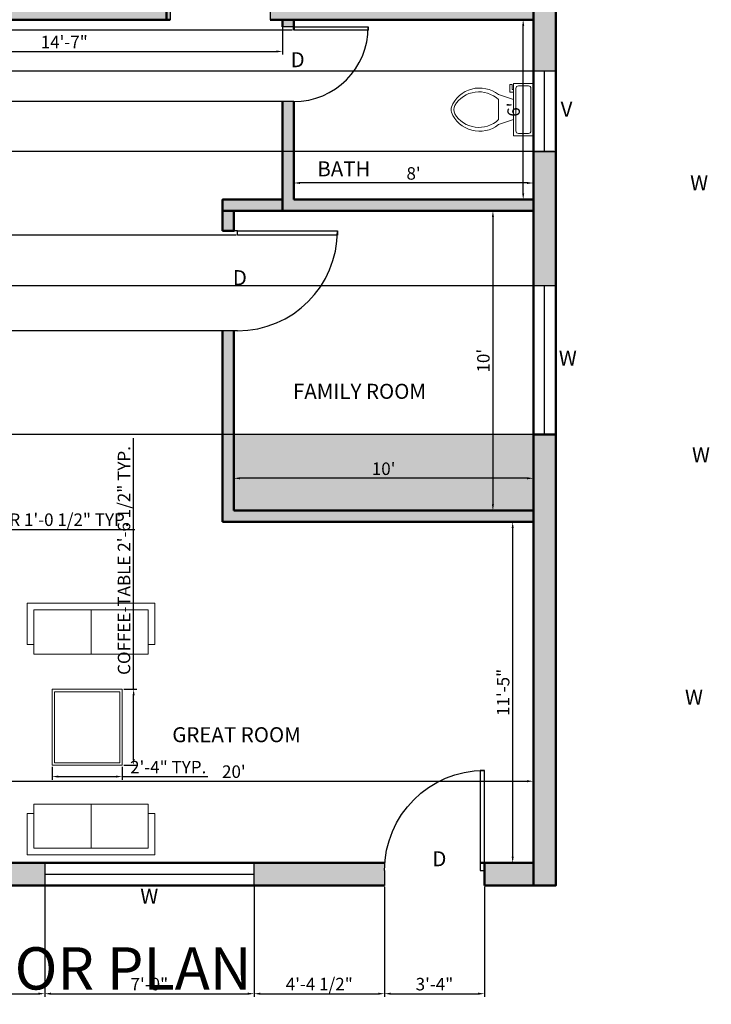
# Model space of a CAD drawing. Units: inches. Extents: x 2064 to 2999, y 1440 to 2089.
# Tile 3 of 7: x 2263 to 2540, y 1440 to 1835. Entities that reach past the tile are written whole.
import ezdxf

# ---------------------------------------------------------------- set-up
doc = ezdxf.new("R2010")
doc.units = ezdxf.units.IN
for name, color, linetype, lineweight in [('A-ANNO-DIMS', 2, 'Continuous', 18), ('A-ANNO-TEXT', 3, 'Continuous', 18), ('A-AREA-IDEN', 7, 'Continuous', 18), ('A-DOOR', 4, 'Continuous', 25), ('A-FLOR-FIXT', 9, 'Continuous', 18), ('A-FURN', 8, 'Continuous', 18), ('A-FURN-PATT', 252, 'Continuous', 13), ('A-GLAZ', 3, 'Continuous', 25), ('A-WALL', 7, 'Continuous', 50), ('A-WALL-PATT', 8, 'Continuous', 13)]:
    doc.layers.add(name, color=color, linetype=linetype, lineweight=lineweight)
doc.styles.get("Standard").update_dxf_attribs({"font": 'arial.ttf'})
doc.dimstyles.new('ISO-25', dxfattribs={"dimtxt": 5, "dimasz": 2.5, "dimexe": 1.25, "dimexo": 0.625, "dimtad": 1, "dimdec": 0, "dimlunit": 4, "dimtxsty": 'Standard', "dimcen": 2.5, "dimadec": 0, "dimazin": 0, "dimtfac": 1, "dimtdec": 0, "dimtmove": 0, "dimatfit": 3, "dimfxl": 1, "dimarcsym": 0})

# ---------------------------------------------------------------- blocks, each defined once
blk = doc.blocks.new('*U2')
for p, q in [((0, 0), (0, -6)), ((40, 0), (40, -6))]:
    blk.add_line(p, q)
blk.add_lwpolyline([(0, 0), (0, 40), (1.75, 40), (1.75, 0)], close=True)
blk.add_arc((0, 0), 40, 0, 90)
blk = doc.blocks.new('*U4')
for p, q in [((9.5, -6), (9.5, -2)), ((-10, -8.5), (-8, -8.5)), ((-10, -9.5), (-10, -8.5)), ((-7, -9.5), (-10, -9.5)), ((-8, -8.5), (-8, -8)), ((-7, -8), (-7, -9.5)), ((-4, -8), (-6, -14)), ((4, -8), (6, -14)), ((4, -14), (-4, -14))]:
    blk.add_line(p, q)
blk.add_lwpolyline([(10.5, -8), (10.5, 0), (-10.5, 0), (-10.5, -8)], close=True)
for points in [[(-9.5, -2), (-9.5, -6)], [(8.5, -1), (-8.5, -1)], [(-8.5, -7), (8.5, -7)]]:
    blk.add_lwpolyline(points)
for centre, radius, start, end in [((-8.62, -1.88), 0.884, 81.8699, 188.1301), ((8.62, -1.88), 0.884, 351.8699, 98.1301), ((-8.62, -6.12), 0.884, 171.8699, 278.1301), ((8.62, -6.12), 0.884, 261.8699, 8.1301), ((3.52, -21.58), 12.17, 141.4691, 247.9714), ((4.2, -21.82), 11.33, 136.3677, 238.9468), ((-3.52, -21.58), 12.17, 292.0284, 38.5307), ((-4.2, -21.82), 11.33, 301.053, 43.6321), ((0, -27.88), 4, 245.7318, 294.2682), ((0, -29), 4, 254.8605, 285.1395)]:
    blk.add_arc(centre, radius, start, end)
blk = doc.blocks.new('*D10')
at = {"layer": 'A-ANNO-DIMS', "color": 0, "lineweight": -2, "transparency": 16777216}
for p, q in [((2468.19, 1834.57), (2463.48, 1834.57)), ((2464.73, 1765.07), (2464.73, 1832.07)), ((2468.19, 1762.57), (2463.48, 1762.57))]:
    blk.add_line(p, q, dxfattribs=at)
at = {"layer": 'A-ANNO-DIMS', "color": 0, "transparency": 16777216}
for points in [[(2464.32, 1832.07), (2465.15, 1832.07), (2464.73, 1834.57)], [(2464.32, 1765.07), (2465.15, 1765.07), (2464.73, 1762.57)]]:
    blk.add_solid(points, dxfattribs=at)
at = {"layer": 'Defpoints', "color": 0, "transparency": 16777216}
for p in [(2464.73, 1834.57), (2468.82, 1834.57), (2468.82, 1762.57)]:
    blk.add_point(p, dxfattribs=at)
at = {"layer": 'A-ANNO-DIMS', "color": 0, "transparency": 16777216, "insert": (2461.55, 1798.57), "char_height": 5, "attachment_point": 5, "rotation": 90}
blk.add_mtext("6'", dxfattribs=at)
blk = doc.blocks.new('*D11')
at = {"layer": 'A-ANNO-DIMS', "color": 0, "lineweight": -2, "transparency": 16777216}
for p, q in [((2372.82, 1763.2), (2372.82, 1770.46)), ((2468.82, 1763.2), (2468.82, 1770.46)), ((2466.32, 1769.21), (2375.32, 1769.21))]:
    blk.add_line(p, q, dxfattribs=at)
at = {"layer": 'A-ANNO-DIMS', "color": 0, "transparency": 16777216}
for points in [[(2375.32, 1769.63), (2375.32, 1768.8), (2372.82, 1769.21)], [(2466.32, 1769.63), (2466.32, 1768.8), (2468.82, 1769.21)]]:
    blk.add_solid(points, dxfattribs=at)
at = {"layer": 'Defpoints', "color": 0, "transparency": 16777216}
for p in [(2372.82, 1769.21), (2372.82, 1762.57), (2468.82, 1762.57)]:
    blk.add_point(p, dxfattribs=at)
at = {"layer": 'A-ANNO-DIMS', "color": 0, "transparency": 16777216, "insert": (2420.82, 1772.39), "char_height": 5, "attachment_point": 5}
blk.add_mtext("8'", dxfattribs=at)
blk = doc.blocks.new('*D12')
at = {"layer": 'A-ANNO-DIMS', "color": 0, "lineweight": -2, "transparency": 16777216}
for p, q in [((2348.82, 1638.7), (2348.82, 1652.27)), ((2468.82, 1638.7), (2468.82, 1652.27)), ((2466.32, 1651.02), (2351.32, 1651.02))]:
    blk.add_line(p, q, dxfattribs=at)
at = {"layer": 'A-ANNO-DIMS', "color": 0, "transparency": 16777216}
for points in [[(2351.32, 1651.43), (2351.32, 1650.6), (2348.82, 1651.02)], [(2466.32, 1651.43), (2466.32, 1650.6), (2468.82, 1651.02)]]:
    blk.add_solid(points, dxfattribs=at)
at = {"layer": 'Defpoints', "color": 0, "transparency": 16777216}
for p in [(2348.82, 1651.02), (2348.82, 1638.07), (2468.82, 1638.07)]:
    blk.add_point(p, dxfattribs=at)
at = {"layer": 'A-ANNO-DIMS', "color": 0, "transparency": 16777216, "insert": (2408.82, 1654.19), "char_height": 5, "attachment_point": 5}
blk.add_mtext("10'", dxfattribs=at)
blk = doc.blocks.new('*D13')
at = {"layer": 'A-ANNO-DIMS', "color": 0, "lineweight": -2, "transparency": 16777216}
for p, q in [((2468.19, 1758.07), (2451.35, 1758.07)), ((2452.6, 1755.57), (2452.6, 1640.57)), ((2468.19, 1638.07), (2451.35, 1638.07))]:
    blk.add_line(p, q, dxfattribs=at)
at = {"layer": 'A-ANNO-DIMS', "color": 0, "transparency": 16777216}
for points in [[(2452.19, 1755.57), (2453.02, 1755.57), (2452.6, 1758.07)], [(2452.19, 1640.57), (2453.02, 1640.57), (2452.6, 1638.07)]]:
    blk.add_solid(points, dxfattribs=at)
at = {"layer": 'Defpoints', "color": 0, "transparency": 16777216}
for p in [(2468.82, 1758.07), (2452.6, 1638.07), (2468.82, 1638.07)]:
    blk.add_point(p, dxfattribs=at)
at = {"layer": 'A-ANNO-DIMS', "color": 0, "transparency": 16777216, "insert": (2449.43, 1698.07), "char_height": 5, "attachment_point": 5, "rotation": 90}
blk.add_mtext("10'", dxfattribs=at)
blk = doc.blocks.new('*D15')
at = {"layer": 'A-ANNO-DIMS', "color": 0, "lineweight": -2, "transparency": 16777216}
for p, q in [((2228.82, 1497.7), (2228.82, 1531.02)), ((2231.32, 1529.77), (2466.32, 1529.77)), ((2468.82, 1497.7), (2468.82, 1531.02))]:
    blk.add_line(p, q, dxfattribs=at)
at = {"layer": 'A-ANNO-DIMS', "color": 0, "transparency": 16777216}
for points in [[(2231.32, 1530.19), (2231.32, 1529.36), (2228.82, 1529.77)], [(2466.32, 1530.19), (2466.32, 1529.36), (2468.82, 1529.77)]]:
    blk.add_solid(points, dxfattribs=at)
at = {"layer": 'Defpoints', "color": 0, "transparency": 16777216}
for p in [(2468.82, 1529.77), (2228.82, 1497.07), (2468.82, 1497.07)]:
    blk.add_point(p, dxfattribs=at)
at = {"layer": 'A-ANNO-DIMS', "color": 0, "transparency": 16777216, "insert": (2348.82, 1532.95), "char_height": 5, "attachment_point": 5}
blk.add_mtext("20'", dxfattribs=at)
blk = doc.blocks.new('*D16')
at = {"layer": 'A-ANNO-DIMS', "color": 0, "lineweight": -2, "transparency": 16777216}
for p, q in [((2193.43, 1833.95), (2193.43, 1820.6)), ((2368.32, 1833.95), (2368.32, 1820.6)), ((2195.93, 1821.85), (2365.82, 1821.85))]:
    blk.add_line(p, q, dxfattribs=at)
at = {"layer": 'A-ANNO-DIMS', "color": 0, "transparency": 16777216}
for points in [[(2195.93, 1822.26), (2195.93, 1821.43), (2193.43, 1821.85)], [(2365.82, 1822.26), (2365.82, 1821.43), (2368.32, 1821.85)]]:
    blk.add_solid(points, dxfattribs=at)
at = {"layer": 'Defpoints', "color": 0, "transparency": 16777216}
for p in [(2193.43, 1834.57), (2368.32, 1834.57), (2368.32, 1821.85)]:
    blk.add_point(p, dxfattribs=at)
at = {"layer": 'A-ANNO-DIMS', "color": 0, "transparency": 16777216, "insert": (2280.88, 1824.98), "char_height": 5, "attachment_point": 5}
blk.add_mtext('14\'-7"', dxfattribs=at)
blk = doc.blocks.new('*D38')
at = {"layer": 'A-ANNO-DIMS', "color": 0, "lineweight": -2, "transparency": 16777216}
for p, q in [((2468.19, 1633.57), (2459.27, 1633.57)), ((2460.52, 1499.57), (2460.52, 1631.07)), ((2468.19, 1497.07), (2459.27, 1497.07))]:
    blk.add_line(p, q, dxfattribs=at)
at = {"layer": 'A-ANNO-DIMS', "color": 0, "transparency": 16777216}
for points in [[(2460.11, 1631.07), (2460.94, 1631.07), (2460.52, 1633.57)], [(2460.11, 1499.57), (2460.94, 1499.57), (2460.52, 1497.07)]]:
    blk.add_solid(points, dxfattribs=at)
at = {"layer": 'Defpoints', "color": 0, "transparency": 16777216}
for p in [(2460.52, 1633.57), (2468.82, 1633.57), (2468.82, 1497.07)]:
    blk.add_point(p, dxfattribs=at)
at = {"layer": 'A-ANNO-DIMS', "color": 0, "transparency": 16777216, "insert": (2457.35, 1565.32), "char_height": 5, "attachment_point": 5, "rotation": 90}
blk.add_mtext('11\'-5"', dxfattribs=at)
blk = doc.blocks.new('SOFA-2')
for p, q in [((25.58, 20.31), (25.58, 2.6)), ((2.71, 16.54), (0, 16.54)), ((0, 16.54), (0, 0)), ((51.13, 16.54), (48.46, 16.54)), ((51.13, 0), (51.13, 16.54)), ((0, 0), (51.13, 0))]:
    blk.add_line(p, q)
blk.add_lwpolyline([(2.71, 2.6), (48.46, 2.6), (48.46, 20.31), (2.71, 20.31)], close=True)
blk = doc.blocks.new('COFFEE-TABLE')
for points in [[(0, 0), (28.15, 0), (28.15, 30.4), (0, 30.4)], [(1, 1), (27.15, 1), (27.15, 29.4), (1, 29.4)]]:
    blk.add_lwpolyline(points, close=True)
blk = doc.blocks.new('WIN-60')
blk.add_line((4.5, 0), (4.5, 59.54))
blk.add_lwpolyline([(0, 0), (9, 0), (9, 59.54), (0, 59.54)], close=True)
blk = doc.blocks.new('*D55')
at = {"layer": 'A-ANNO-DIMS', "color": 0, "lineweight": -2, "transparency": 16777216}
for p, q in [((2308.68, 1566.59), (2308.68, 1667.13)), ((2304.75, 1566.59), (2309.93, 1566.59)), ((2308.68, 1538.68), (2308.68, 1564.09)), ((2304.75, 1536.18), (2309.93, 1536.18))]:
    blk.add_line(p, q, dxfattribs=at)
at = {"layer": 'A-ANNO-DIMS', "color": 0, "transparency": 16777216}
for points in [[(2308.27, 1564.09), (2309.1, 1564.09), (2308.68, 1566.59)], [(2308.27, 1538.68), (2309.1, 1538.68), (2308.68, 1536.18)]]:
    blk.add_solid(points, dxfattribs=at)
at = {"layer": 'Defpoints', "color": 0, "transparency": 16777216}
for p in [(2304.12, 1566.59), (2308.68, 1566.59), (2304.12, 1536.18)]:
    blk.add_point(p, dxfattribs=at)
at = {"layer": 'A-ANNO-DIMS', "color": 0, "transparency": 16777216, "insert": (2305.47, 1618.11), "char_height": 5, "attachment_point": 5, "rotation": 90}
blk.add_mtext('COFFEE-TABLE 2\'-6 1/2" TYP.', dxfattribs=at)
blk = doc.blocks.new('*D56')
at = {"layer": 'A-ANNO-DIMS', "color": 0, "lineweight": -2, "transparency": 16777216}
for p, q in [((2275.98, 1535.56), (2275.98, 1530.37)), ((2304.12, 1535.56), (2304.12, 1530.37)), ((2278.48, 1531.62), (2301.62, 1531.62)), ((2304.12, 1531.62), (2338.44, 1531.62))]:
    blk.add_line(p, q, dxfattribs=at)
at = {"layer": 'A-ANNO-DIMS', "color": 0, "transparency": 16777216}
for points in [[(2278.48, 1532.04), (2278.48, 1531.21), (2275.98, 1531.62)], [(2301.62, 1532.04), (2301.62, 1531.21), (2304.12, 1531.62)]]:
    blk.add_solid(points, dxfattribs=at)
at = {"layer": 'Defpoints', "color": 0, "transparency": 16777216}
for p in [(2275.98, 1536.18), (2304.12, 1536.18), (2304.12, 1531.62)]:
    blk.add_point(p, dxfattribs=at)
at = {"layer": 'A-ANNO-DIMS', "color": 0, "transparency": 16777216, "insert": (2322.53, 1534.76), "char_height": 5, "attachment_point": 5}
blk.add_mtext('2\'-4" TYP.', dxfattribs=at)
blk = doc.blocks.new('*D57')
at = {"layer": 'A-ANNO-DIMS', "color": 0, "lineweight": -2, "transparency": 16777216}
for p, q in [((2200.61, 1631.83), (2200.61, 1629.33)), ((2213.15, 1631.83), (2213.15, 1629.33)), ((2203.11, 1630.58), (2210.65, 1630.58)), ((2213.15, 1630.58), (2309.22, 1630.58))]:
    blk.add_line(p, q, dxfattribs=at)
at = {"layer": 'A-ANNO-DIMS', "color": 0, "transparency": 16777216}
for points in [[(2203.11, 1631), (2203.11, 1630.16), (2200.61, 1630.58)], [(2210.65, 1631), (2210.65, 1630.16), (2213.15, 1630.58)]]:
    blk.add_solid(points, dxfattribs=at)
at = {"layer": 'Defpoints', "color": 0, "transparency": 16777216}
for p in [(2200.61, 1632.46), (2213.15, 1632.46), (2213.15, 1630.58)]:
    blk.add_point(p, dxfattribs=at)
at = {"layer": 'A-ANNO-DIMS', "color": 0, "transparency": 16777216, "insert": (2262.43, 1633.79), "char_height": 5, "attachment_point": 5}
blk.add_mtext('DINING-CHAIR 1\'-0 1/2" TYP.', dxfattribs=at)
blk = doc.blocks.new('*D70')
at = {"layer": 'A-ANNO-DIMS', "color": 0, "lineweight": -2, "transparency": 16777216}
for p, q in [((2477.19, 1865.66), (2073.22, 1865.66)), ((2074.47, 1863.16), (2074.47, 1816.51)), ((2477.19, 1814.01), (2073.22, 1814.01))]:
    blk.add_line(p, q, dxfattribs=at)
at = {"layer": 'A-ANNO-DIMS', "color": 0, "transparency": 16777216}
for points in [[(2074.05, 1863.16), (2074.89, 1863.16), (2074.47, 1865.66)], [(2074.05, 1816.51), (2074.89, 1816.51), (2074.47, 1814.01)]]:
    blk.add_solid(points, dxfattribs=at)
at = {"layer": 'Defpoints', "color": 0, "transparency": 16777216}
for p in [(2477.82, 1865.66), (2074.47, 1814.01), (2477.82, 1814.01)]:
    blk.add_point(p, dxfattribs=at)
at = {"layer": 'A-ANNO-DIMS', "color": 0, "transparency": 16777216, "insert": (2071.26, 1839.83), "char_height": 5, "attachment_point": 5, "rotation": 90}
blk.add_mtext('4\'-3 1/2"', dxfattribs=at)
blk = doc.blocks.new('*D71')
at = {"layer": 'A-ANNO-DIMS', "color": 0, "lineweight": -2, "transparency": 16777216}
for p, q in [((2477.19, 1814.01), (2073.22, 1814.01)), ((2074.47, 1811.51), (2074.47, 1784.3)), ((2477.19, 1781.8), (2073.22, 1781.8))]:
    blk.add_line(p, q, dxfattribs=at)
at = {"layer": 'A-ANNO-DIMS', "color": 0, "transparency": 16777216}
for points in [[(2074.05, 1811.51), (2074.89, 1811.51), (2074.47, 1814.01)], [(2074.05, 1784.3), (2074.89, 1784.3), (2074.47, 1781.8)]]:
    blk.add_solid(points, dxfattribs=at)
at = {"layer": 'Defpoints', "color": 0, "transparency": 16777216}
for p in [(2477.82, 1814.01), (2074.47, 1781.8), (2477.82, 1781.8)]:
    blk.add_point(p, dxfattribs=at)
at = {"layer": 'A-ANNO-DIMS', "color": 0, "transparency": 16777216, "insert": (2071.29, 1797.91), "char_height": 5, "attachment_point": 5, "rotation": 90}
blk.add_mtext('2\'-8"', dxfattribs=at)
blk = doc.blocks.new('*D72')
at = {"layer": 'A-ANNO-DIMS', "color": 0, "lineweight": -2, "transparency": 16777216}
for p, q in [((2477.19, 1781.8), (2073.22, 1781.8)), ((2074.47, 1779.3), (2074.47, 1730.57)), ((2477.19, 1728.07), (2073.22, 1728.07))]:
    blk.add_line(p, q, dxfattribs=at)
at = {"layer": 'A-ANNO-DIMS', "color": 0, "transparency": 16777216}
for points in [[(2074.05, 1779.3), (2074.89, 1779.3), (2074.47, 1781.8)], [(2074.05, 1730.57), (2074.89, 1730.57), (2074.47, 1728.07)]]:
    blk.add_solid(points, dxfattribs=at)
at = {"layer": 'Defpoints', "color": 0, "transparency": 16777216}
for p in [(2477.82, 1781.8), (2074.47, 1728.07), (2477.82, 1728.07)]:
    blk.add_point(p, dxfattribs=at)
at = {"layer": 'A-ANNO-DIMS', "color": 0, "transparency": 16777216, "insert": (2071.26, 1754.94), "char_height": 5, "attachment_point": 5, "rotation": 90}
blk.add_mtext('4\'-5 1/2"', dxfattribs=at)
blk = doc.blocks.new('*D73')
at = {"layer": 'A-ANNO-DIMS', "color": 0, "lineweight": -2, "transparency": 16777216}
for p, q in [((2477.19, 1728.07), (2073.22, 1728.07)), ((2074.47, 1725.57), (2074.47, 1671.03)), ((2477.19, 1668.53), (2073.22, 1668.53))]:
    blk.add_line(p, q, dxfattribs=at)
at = {"layer": 'A-ANNO-DIMS', "color": 0, "transparency": 16777216}
for points in [[(2074.05, 1725.57), (2074.89, 1725.57), (2074.47, 1728.07)], [(2074.05, 1671.03), (2074.89, 1671.03), (2074.47, 1668.53)]]:
    blk.add_solid(points, dxfattribs=at)
at = {"layer": 'Defpoints', "color": 0, "transparency": 16777216}
for p in [(2477.82, 1728.07), (2074.47, 1668.53), (2477.82, 1668.53)]:
    blk.add_point(p, dxfattribs=at)
at = {"layer": 'A-ANNO-DIMS', "color": 0, "transparency": 16777216, "insert": (2071.26, 1698.3), "char_height": 5, "attachment_point": 5, "rotation": 90}
blk.add_mtext('4\'-11 1/2"', dxfattribs=at)
blk = doc.blocks.new('*D78')
at = {"layer": 'A-ANNO-DIMS', "color": 0, "lineweight": -2, "transparency": 16777216}
for p, q in [((2117.82, 1487.45), (2117.82, 1443.47)), ((2273.05, 1487.45), (2273.05, 1443.47)), ((2120.32, 1444.72), (2270.55, 1444.72))]:
    blk.add_line(p, q, dxfattribs=at)
at = {"layer": 'A-ANNO-DIMS', "color": 0, "transparency": 16777216}
for points in [[(2120.32, 1445.14), (2120.32, 1444.3), (2117.82, 1444.72)], [(2270.55, 1445.14), (2270.55, 1444.3), (2273.05, 1444.72)]]:
    blk.add_solid(points, dxfattribs=at)
at = {"layer": 'Defpoints', "color": 0, "transparency": 16777216}
for p in [(2117.82, 1488.07), (2273.05, 1488.07), (2273.05, 1444.72)]:
    blk.add_point(p, dxfattribs=at)
at = {"layer": 'A-ANNO-DIMS', "color": 0, "transparency": 16777216, "insert": (2195.43, 1447.86), "char_height": 5, "attachment_point": 5}
blk.add_mtext('12\'-11"', dxfattribs=at)
blk = doc.blocks.new('*D79')
at = {"layer": 'A-ANNO-DIMS', "color": 0, "lineweight": -2, "transparency": 16777216}
for p, q in [((2273.05, 1487.45), (2273.05, 1443.47)), ((2356.92, 1487.45), (2356.92, 1443.47)), ((2275.55, 1444.72), (2354.42, 1444.72))]:
    blk.add_line(p, q, dxfattribs=at)
at = {"layer": 'A-ANNO-DIMS', "color": 0, "transparency": 16777216}
for points in [[(2275.55, 1445.14), (2275.55, 1444.3), (2273.05, 1444.72)], [(2354.42, 1445.14), (2354.42, 1444.3), (2356.92, 1444.72)]]:
    blk.add_solid(points, dxfattribs=at)
at = {"layer": 'Defpoints', "color": 0, "transparency": 16777216}
for p in [(2273.05, 1488.07), (2356.92, 1488.07), (2356.92, 1444.72)]:
    blk.add_point(p, dxfattribs=at)
at = {"layer": 'A-ANNO-DIMS', "color": 0, "transparency": 16777216, "insert": (2314.98, 1447.9), "char_height": 5, "attachment_point": 5}
blk.add_mtext('7\'-0"', dxfattribs=at)
blk = doc.blocks.new('*D80')
at = {"layer": 'A-ANNO-DIMS', "color": 0, "lineweight": -2, "transparency": 16777216}
for p, q in [((2356.92, 1487.45), (2356.92, 1443.47)), ((2409.19, 1487.45), (2409.19, 1443.47)), ((2359.42, 1444.72), (2406.69, 1444.72))]:
    blk.add_line(p, q, dxfattribs=at)
at = {"layer": 'A-ANNO-DIMS', "color": 0, "transparency": 16777216}
for points in [[(2359.42, 1445.14), (2359.42, 1444.3), (2356.92, 1444.72)], [(2406.69, 1445.14), (2406.69, 1444.3), (2409.19, 1444.72)]]:
    blk.add_solid(points, dxfattribs=at)
at = {"layer": 'Defpoints', "color": 0, "transparency": 16777216}
for p in [(2356.92, 1488.07), (2409.19, 1488.07), (2409.19, 1444.72)]:
    blk.add_point(p, dxfattribs=at)
at = {"layer": 'A-ANNO-DIMS', "color": 0, "transparency": 16777216, "insert": (2383.05, 1447.93), "char_height": 5, "attachment_point": 5}
blk.add_mtext('4\'-4 1/2"', dxfattribs=at)
blk = doc.blocks.new('*D81')
at = {"layer": 'A-ANNO-DIMS', "color": 0, "lineweight": -2, "transparency": 16777216}
for p, q in [((2409.19, 1487.45), (2409.19, 1443.47)), ((2449.19, 1487.45), (2449.19, 1443.47)), ((2411.69, 1444.72), (2446.69, 1444.72))]:
    blk.add_line(p, q, dxfattribs=at)
at = {"layer": 'A-ANNO-DIMS', "color": 0, "transparency": 16777216}
for points in [[(2411.69, 1445.14), (2411.69, 1444.3), (2409.19, 1444.72)], [(2446.69, 1445.14), (2446.69, 1444.3), (2449.19, 1444.72)]]:
    blk.add_solid(points, dxfattribs=at)
at = {"layer": 'Defpoints', "color": 0, "transparency": 16777216}
for p in [(2409.19, 1488.07), (2449.19, 1488.07), (2449.19, 1444.72)]:
    blk.add_point(p, dxfattribs=at)
at = {"layer": 'A-ANNO-DIMS', "color": 0, "transparency": 16777216, "insert": (2429.19, 1447.9), "char_height": 5, "attachment_point": 5}
blk.add_mtext('3\'-4"', dxfattribs=at)
blk = doc.blocks.new('*D113')
at = {"layer": 'A-ANNO-DIMS', "color": 0, "lineweight": -2, "transparency": 16777216}
for p, q in [((2372.19, 1830.37), (2073.22, 1830.37)), ((2074.47, 1827.87), (2074.47, 1804.28)), ((2372.19, 1801.78), (2073.22, 1801.78))]:
    blk.add_line(p, q, dxfattribs=at)
at = {"layer": 'A-ANNO-DIMS', "color": 0, "transparency": 16777216}
for points in [[(2074.05, 1827.87), (2074.89, 1827.87), (2074.47, 1830.37)], [(2074.05, 1804.28), (2074.89, 1804.28), (2074.47, 1801.78)]]:
    blk.add_solid(points, dxfattribs=at)
at = {"layer": 'Defpoints', "color": 0, "transparency": 16777216}
for p in [(2372.82, 1830.37), (2074.47, 1801.78), (2372.82, 1801.78)]:
    blk.add_point(p, dxfattribs=at)
at = {"layer": 'A-ANNO-DIMS', "color": 0, "transparency": 16777216, "insert": (2071.26, 1816.07), "char_height": 5, "attachment_point": 5, "rotation": 90}
blk.add_mtext('2\'-4 1/2"', dxfattribs=at)
blk = doc.blocks.new('*D114')
at = {"layer": 'A-ANNO-DIMS', "color": 0, "lineweight": -2, "transparency": 16777216}
for p, q in [((2349.69, 1748.3), (2073.22, 1748.3)), ((2074.47, 1745.8), (2074.47, 1712.55)), ((2348.19, 1710.05), (2073.22, 1710.05))]:
    blk.add_line(p, q, dxfattribs=at)
at = {"layer": 'A-ANNO-DIMS', "color": 0, "transparency": 16777216}
for points in [[(2074.05, 1745.8), (2074.89, 1745.8), (2074.47, 1748.3)], [(2074.05, 1712.55), (2074.89, 1712.55), (2074.47, 1710.05)]]:
    blk.add_solid(points, dxfattribs=at)
at = {"layer": 'Defpoints', "color": 0, "transparency": 16777216}
for p in [(2350.32, 1748.3), (2074.47, 1710.05), (2348.82, 1710.05)]:
    blk.add_point(p, dxfattribs=at)
at = {"layer": 'A-ANNO-DIMS', "color": 0, "transparency": 16777216, "insert": (2071.26, 1729.18), "char_height": 5, "attachment_point": 5, "rotation": 90}
blk.add_mtext('3\'-2 1/2"', dxfattribs=at)

msp = doc.modelspace()

# ---------------------------------------------------------------- hatches: boundary and pattern name
at = {"layer": 'A-FURN-PATT'}
h = msp.add_hatch(color=256, dxfattribs=at)
h.dxf.hatch_style = 1
h.paths.add_polyline_path([(2211.98, 1959.07), (2126.82, 1959.07), (2126.82, 1938.57), (2211.98, 1938.57)])
h.paths.add_polyline_path([(2669.87, 1959.07), (2646.96, 1959.07), (2646.96, 1892.49), (2669.87, 1892.49)])
h.paths.add_polyline_path([(2468.82, 1668.53), (2348.82, 1668.53), (2348.82, 1638.07), (2468.82, 1638.07)])
h.paths.add_polyline_path([(2891.87, 1667.99), (2780.13, 1667.99), (2780.13, 1638.07), (2891.87, 1638.07)])
h.paths.add_polyline_path([(2854.27, 1658.75), (2854.27, 1650.97), (2859.31, 1650.97), (2859.31, 1658.75), (2862.16, 1658.75), (2862.16, 1650.97), (2867.47, 1650.97), (2867.47, 1658.75), (2870.33, 1658.75), (2870.33, 1650.97), (2879.45, 1650.97), (2879.45, 1658.75), (2882.31, 1658.75), (2882.31, 1643.24), (2879.45, 1643.24), (2879.45, 1650.97), (2870.33, 1650.97), (2870.33, 1643.24), (2867.47, 1643.24), (2867.47, 1650.97), (2862.16, 1650.97), (2862.16, 1643.24), (2859.31, 1643.24), (2859.31, 1650.97), (2854.27, 1650.97), (2854.27, 1643.24), (2851.41, 1643.24), (2851.41, 1650.97), (2845.97, 1650.97), (2845.97, 1643.24), (2843.11, 1643.24), (2843.11, 1650.97), (2839.98, 1650.97), (2839.98, 1643.24), (2837.12, 1643.24), (2837.12, 1650.97), (2831.27, 1650.97), (2831.27, 1643.24), (2828.41, 1643.24), (2828.41, 1650.97), (2823.78, 1650.97), (2823.78, 1643.24), (2820.92, 1643.24), (2820.92, 1650.97), (2816.56, 1650.97), (2816.56, 1641.66), (2813.71, 1641.66), (2813.71, 1650.97), (2808.81, 1650.97), (2808.81, 1641.66), (2805.95, 1641.66), (2805.95, 1650.97), (2801.73, 1650.97), (2801.73, 1641.66), (2798.87, 1641.66), (2798.87, 1650.97), (2794.92, 1650.97), (2794.92, 1643.24), (2792.06, 1643.24), (2792.06, 1658.75), (2794.92, 1658.75), (2794.92, 1650.97), (2798.87, 1650.97), (2798.87, 1657.16), (2801.73, 1657.16), (2801.73, 1650.97), (2805.95, 1650.97), (2805.95, 1657.16), (2808.81, 1657.16), (2808.81, 1650.97), (2813.71, 1650.97), (2813.71, 1657.16), (2816.56, 1657.16), (2816.56, 1650.97), (2820.92, 1650.97), (2820.92, 1658.75), (2823.78, 1658.75), (2823.78, 1650.97), (2828.41, 1650.97), (2828.41, 1658.75), (2831.27, 1658.75), (2831.27, 1650.97), (2837.12, 1650.97), (2837.12, 1658.75), (2839.98, 1658.75), (2839.98, 1650.97), (2843.11, 1650.97), (2843.11, 1658.75), (2845.97, 1658.75), (2845.97, 1650.97), (2851.41, 1650.97), (2851.41, 1658.75)], flags=16)
h.paths.add_polyline_path([(2665.84, 1899.31), (2665.84, 1951.8), (2653.45, 1951.8), (2653.45, 1899.31)], flags=24)
h.paths.add_polyline_path([(2565.91, 1921.55), (2649.69, 1921.55), (2649.69, 1933.95), (2565.91, 1933.95)], flags=9)
h.paths.add_polyline_path([(2402.8, 1649), (2414.4, 1649), (2414.4, 1659.3), (2402.8, 1659.3)], flags=24)
at = {"layer": 'A-WALL-PATT'}
h = msp.add_hatch(color=256, dxfattribs=at)
h.dxf.hatch_style = 1
h.paths.add_polyline_path([(2267.27, 1968.07), (2215.88, 1968.07), (2215.88, 1959.07), (2246.82, 1959.07), (2267.27, 1959.07)])
h.paths.add_polyline_path([(2477.82, 1968.07), (2300.73, 1968.07), (2300.73, 1959.07), (2317.32, 1959.07), (2468.82, 1959.07), (2468.82, 1925.2), (2477.82, 1925.2)])
h.paths.add_polyline_path([(2154.1, 1968.07), (2117.82, 1968.07), (2117.82, 1784.53), (2126.82, 1784.53), (2126.82, 1959.07), (2154.1, 1959.07)])
h.paths.add_polyline_path([(2126.82, 1716.1), (2117.82, 1716.1), (2117.82, 1685.76), (2126.82, 1685.76)])
h.paths.add_polyline_path([(2126.82, 1617.33), (2117.82, 1617.33), (2117.82, 1589.89), (2126.82, 1589.89)])
h.paths.add_polyline_path([(2273.05, 1497.07), (2228.82, 1497.07), (2126.82, 1497.07), (2126.82, 1521.07), (2126.82, 1521.46), (2117.82, 1521.46), (2117.82, 1488.07), (2273.05, 1488.07)])
h.paths.add_polyline_path([(2409.19, 1494.07, -0.01877), (2409.3, 1497.07), (2356.92, 1497.07), (2356.92, 1488.07), (2409.19, 1488.07)])
h.paths.add_polyline_path([(2468.82, 1638.07), (2348.82, 1638.07), (2348.82, 1668.53), (2348.82, 1710.05), (2344.32, 1710.05), (2344.32, 1633.57), (2468.82, 1633.57)])
h.paths.add_polyline_path([(2228.82, 1567.84), (2224.32, 1567.84), (2224.32, 1497.07), (2228.82, 1497.07)])
h.paths.add_polyline_path([(2477.82, 1781.8), (2468.82, 1781.8), (2468.82, 1762.57), (2468.82, 1728.07), (2477.82, 1728.07)])
h.paths.add_polyline_path([(2468.82, 1762.57), (2372.82, 1762.57), (2372.82, 1801.78), (2368.32, 1801.78), (2368.32, 1758.07), (2468.82, 1758.07)])
h.paths.add_polyline_path([(2477.82, 1865.66), (2468.82, 1865.66), (2468.82, 1814.01), (2477.82, 1814.01)])
h.paths.add_polyline_path([(2321.82, 1959.07), (2317.32, 1959.07), (2317.32, 1839.07), (2251.32, 1839.07), (2251.32, 1834.57), (2321.82, 1834.57)])
h.paths.add_polyline_path([(2200.07, 1839.07), (2126.82, 1839.07), (2126.82, 1834.57), (2200.07, 1834.57)])
h.paths.add_polyline_path([(2193.43, 1834.57), (2188.93, 1834.57), (2188.93, 1710.22), (2193.43, 1710.22)])
h.paths.add_polyline_path([(2251.32, 1959.07), (2246.82, 1959.07), (2246.82, 1950.75), (2251.21, 1950.75), (2251.32, 1950.75)])
h.paths.add_polyline_path([(2251.32, 1921.46), (2246.82, 1921.46), (2246.82, 1839.07), (2240.07, 1839.07), (2240.07, 1834.57), (2251.32, 1834.57), (2251.32, 1839.07)])
h.paths.add_polyline_path([(2468.82, 1839.07), (2363.36, 1839.07), (2363.36, 1834.57), (2468.82, 1834.57)])
h.paths.add_polyline_path([(2323.36, 1839.07), (2321.82, 1839.07), (2321.82, 1834.57), (2323.36, 1834.57)])
h = msp.add_hatch(color=256, dxfattribs=at)
h.dxf.hatch_style = 1
h.paths.add_polyline_path([(2449.19, 1497.07), (2449.19, 1494.07), (2449.19, 1488.07), (2468.82, 1488.07), (2468.82, 1497.07)])
h.paths.add_polyline_path([(2468.82, 1488.07), (2477.82, 1488.07), (2477.82, 1668.53), (2468.82, 1668.53)])
h.paths.add_polyline_path([(2454.62, 1692.05), (2454.62, 1703.66), (2444.32, 1703.66), (2444.32, 1692.05)], flags=9)
h.paths.add_polyline_path([(2167.39, 1527.81), (2183.8, 1527.81), (2183.8, 1538.12), (2167.39, 1538.12)], flags=9)
h.paths.add_polyline_path([(2343.08, 1527.75), (2354.68, 1527.75), (2354.68, 1538.06), (2343.08, 1538.06)], flags=9)
h.paths.add_polyline_path([(2462.54, 1554.96), (2462.54, 1575.25), (2452.24, 1575.25), (2452.24, 1554.96)], flags=9)
h.paths.add_polyline_path([(2140.63, 1624.84), (2140.63, 1645.13), (2130.32, 1645.13), (2130.32, 1624.84)], flags=9)
h.paths.add_polyline_path([(2137.9, 1938.01), (2190.4, 1938.01), (2190.4, 1950.4), (2137.9, 1950.4)], flags=9)
h.paths.add_polyline_path([(2337.44, 1898.9), (2337.44, 1951.39), (2325.04, 1951.39), (2325.04, 1898.9)], flags=9)
h.paths.add_polyline_path([(2380.15, 1768.58), (2405.57, 1768.58), (2405.57, 1780.97), (2380.15, 1780.97)], flags=9)
h.paths.add_polyline_path([(2370.32, 1679.42), (2432.16, 1679.42), (2432.16, 1691.82), (2370.32, 1691.82)], flags=9)
h.paths.add_polyline_path([(2322.2, 1541.98), (2382.63, 1541.98), (2382.63, 1554.37), (2322.2, 1554.37)], flags=9)
h.paths.add_polyline_path([(2153.83, 1534.75), (2193.72, 1534.75), (2193.72, 1547.14), (2153.83, 1547.14)], flags=9)
h.paths.add_polyline_path([(2162.47, 1614.19), (2217.78, 1614.19), (2217.78, 1626.58), (2162.47, 1626.58)], flags=9)
h.paths.add_polyline_path([(2217.9, 1723.52), (2261.07, 1723.52), (2261.07, 1735.92), (2217.9, 1735.92)], flags=9)
h.paths.add_polyline_path([(2270.61, 1869.16), (2296.03, 1869.16), (2296.03, 1881.55), (2270.61, 1881.55)], flags=9)
h.paths.add_polyline_path([(2353.7, 1922), (2422.07, 1922), (2422.07, 1934.4), (2353.7, 1934.4)], flags=9)
h.paths.add_polyline_path([(2133.7, 1917.44), (2217.48, 1917.44), (2217.48, 1929.83), (2133.7, 1929.83)], flags=9)
h = msp.add_hatch(color=256, dxfattribs=at)
h.dxf.hatch_style = 1
h.paths.add_polyline_path([(2368.32, 1762.57), (2344.32, 1762.57), (2344.32, 1758.07), (2368.32, 1758.07)])
h.paths.add_polyline_path([(2348.82, 1758.07), (2344.32, 1758.07), (2344.32, 1750.05), (2348.82, 1750.05)])
h.paths.add_polyline_path([(2372.82, 1834.57), (2368.32, 1834.57), (2368.32, 1831.67), (2372.82, 1831.67)])

# ---------------------------------------------------------------- linework, layer by layer
at = {"layer": 'A-FURN'}
msp.add_lwpolyline([(2348.82, 1638.07), (2468.82, 1638.07), (2468.82, 1668.53), (2348.82, 1668.53)], close=True, dxfattribs=at)
at = {"layer": 'A-GLAZ'}
for p, q in [((2473.32, 1781.8), (2473.32, 1814.01)), ((2273.05, 1492.57), (2356.92, 1492.57))]:
    msp.add_line(p, q, dxfattribs=at)
for points in [[(2468.82, 1781.8), (2477.82, 1781.8), (2477.82, 1814.01), (2468.82, 1814.01)], [(2273.05, 1488.07), (2356.92, 1488.07), (2356.92, 1497.07), (2273.05, 1497.07)]]:
    msp.add_lwpolyline(points, close=True, dxfattribs=at)
at = {"layer": 'A-WALL'}
for p, q in [((2477.82, 1968.07), (2477.82, 1488.07)), ((2321.82, 1959.07), (2321.82, 1834.57)), ((2321.82, 1834.57), (2251.32, 1834.57)), ((2321.82, 1834.57), (2323.36, 1834.57)), ((2363.36, 1834.57), (2468.82, 1834.57)), ((2368.32, 1831.67), (2368.32, 1834.57)), ((2372.82, 1830.37), (2372.82, 1834.57)), ((2468.82, 1834.57), (2468.82, 1762.57)), ((2368.32, 1758.07), (2368.32, 1801.78)), ((2372.82, 1762.57), (2372.82, 1801.78)), ((2344.32, 1762.57), (2368.32, 1762.57)), ((2344.32, 1750.05), (2344.32, 1762.57)), ((2468.82, 1762.57), (2372.82, 1762.57)), ((2348.82, 1758.07), (2368.32, 1758.07)), ((2348.82, 1750.05), (2348.82, 1758.07)), ((2468.82, 1758.07), (2368.32, 1758.07)), ((2468.82, 1758.07), (2468.82, 1638.07)), ((2344.32, 1633.57), (2344.32, 1710.05)), ((2348.82, 1638.07), (2348.82, 1710.05)), ((2468.82, 1638.07), (2348.82, 1638.07)), ((2468.82, 1633.57), (2344.32, 1633.57)), ((2409.3, 1497.07), (2228.82, 1497.07)), ((2468.82, 1497.07), (2447.44, 1497.07)), ((2409.19, 1488.07), (2117.82, 1488.07)), ((2477.82, 1488.07), (2449.19, 1488.07))]:
    msp.add_line(p, q, dxfattribs=at)
for points in [[(2449.19, 1488.07), (2477.82, 1488.07), (2477.82, 1968.07), (2117.82, 1968.07), (2117.82, 1488.07), (2409.19, 1488.07)], [(2447.44, 1497.07), (2468.82, 1497.07), (2468.82, 1959.07), (2126.82, 1959.07), (2126.82, 1497.07), (2409.3, 1497.07)]]:
    msp.add_lwpolyline(points, dxfattribs=at)
for points in [[(2344.32, 1758.07), (2368.32, 1758.07), (2368.32, 1762.57), (2344.32, 1762.57)], [(2344.32, 1750.05), (2348.82, 1750.05), (2348.82, 1758.07), (2344.32, 1758.07)], [(2468.82, 1668.53), (2477.82, 1668.53), (2477.82, 1488.07), (2468.82, 1488.07)], [(2449.19, 1488.07), (2468.82, 1488.07), (2468.82, 1497.07), (2449.19, 1497.07)]]:
    msp.add_lwpolyline(points, close=True, dxfattribs=at)

# ---------------------------------------------------------------- block references
at = {"layer": 'A-DOOR'}
msp.add_blockref('*U2', (2323.36, 1840.57), dxfattribs=at)
at = {"layer": 'A-DOOR', "xscale": 0.747418982688762, "yscale": 0.747418982688762, "zscale": 0.747418982688762, "rotation": 270}
msp.add_blockref('*U2', (2372.8, 1831.67), dxfattribs=at)
at = {"layer": 'A-DOOR', "rotation": 270}
msp.add_blockref('*U2', (2350.32, 1750.05), dxfattribs=at)
at = {"layer": 'A-DOOR', "xscale": -1}
msp.add_blockref('*U2', (2449.19, 1494.07), dxfattribs=at)
at = {"layer": 'A-FLOR-FIXT', "rotation": 270}
msp.add_blockref('*U4', (2468.82, 1798.57), dxfattribs=at)
at = {"layer": 'A-FURN', "extrusion": (0, 0, -1), "zscale": -1, "rotation": 180}
msp.add_blockref('SOFA-2', (-2266.04, 1600.99), dxfattribs=at)
at = {"layer": 'A-FURN'}
for name, p in [('COFFEE-TABLE', (2275.98, 1536.18)), ('SOFA-2', (2266.04, 1500.32))]:
    msp.add_blockref(name, p, dxfattribs=at)
at = {"layer": 'A-GLAZ'}
msp.add_blockref('WIN-60', (2468.82, 1668.53), dxfattribs=at)

# ---------------------------------------------------------------- texts
at = {"layer": 'A-ANNO-TEXT', "attachment_point": 1}
for s, width, gutter_width, heights, insert, char_height in [('D', 152.6727, 30.08, [0], (2371.55, 1821.57), 6.02), ('V', 152.6727, 30.08, [0], (2479.73, 1801.76), 6.02), ('W', 152.6727, 30.08, [0], (2531.61, 1772.33), 6.02), ('D', 152.6727, 30.08, [0], (2348.41, 1734.32), 6.02), ('W', 152.6727, 30.08, [0], (2479.01, 1702.16), 6.02), ('W', 152.6727, 30.08, [0], (2532.35, 1663.45), 6.02), ('W', 152.6727, 30.08, [0], (2529.54, 1566.41), 6.02), ('D', 152.6727, 30.08, [0], (2428.33, 1501.73), 6.02), ('W', 152.6727, 30.08, [0], (2311.33, 1486.77), 6.02), ('GROUND FLOOR PLAN', 429.6774, 84.65, [17.52], (2116.47, 1463.31), 16.9292)]:
    msp.add_mtext_dynamic_manual_height_columns(s, width=width, gutter_width=gutter_width, heights=heights, dxfattribs=dict(at, insert=insert, char_height=char_height))
at = {"layer": 'A-AREA-IDEN', "attachment_point": 1}
for s, insert, char_height in [('BATH', (2382.27, 1777.88), 6.015), ('FAMILY ROOM', (2372.52, 1688.83), 6.0153), ('GREAT ROOM', (2324.15, 1551.39), 6.015)]:
    msp.add_mtext_dynamic_manual_height_columns(s, width=152.6727, gutter_width=30.08, heights=[0], dxfattribs=dict(at, insert=insert, char_height=char_height))

# ---------------------------------------------------------------- dimensions: what is measured, and where the dimension line sits
at = {"layer": 'A-ANNO-DIMS'}
for base, p1, p2, override, picture, middle in [((2074.4687, 1814.0143), (2477.8187, 1865.6554), (2477.8187, 1814.0143), {"dimdec": 1, "dimlfac": 1, "dimrnd": 0, "dimzin": 1, "dimdsep": 46, "dimlunit": 4, "dimfrac": 2}, '*D70', (2071.2567, 1839.8348)), ((2464.73, 1834.57), (2468.82, 1762.57), (2468.82, 1834.57), {"dimclrd": 0, "dimclre": 0, "dimclrt": 0}, '*D10', (2461.55, 1798.57)), ((2074.47, 1801.78), (2372.82, 1830.37), (2372.82, 1801.78), {"dimdec": 1, "dimlfac": 1, "dimrnd": 0, "dimzin": 1, "dimdsep": 46, "dimlunit": 4, "dimfrac": 2}, '*D113', (2071.26, 1816.07)), ((2074.47, 1781.8), (2477.82, 1814.01), (2477.82, 1781.8), {"dimdec": 1, "dimlfac": 1, "dimrnd": 0, "dimzin": 1, "dimdsep": 46, "dimlunit": 4, "dimfrac": 2}, '*D71', (2071.29, 1797.91)), ((2074.47, 1728.07), (2477.82, 1781.8), (2477.82, 1728.07), {"dimdec": 1, "dimlfac": 1, "dimrnd": 0, "dimzin": 1, "dimdsep": 46, "dimlunit": 4, "dimfrac": 2}, '*D72', (2071.26, 1754.94)), ((2452.6, 1638.07), (2468.82, 1758.07), (2468.82, 1638.07), {"dimclrd": 0, "dimclre": 0, "dimclrt": 0}, '*D13', (2449.43, 1698.07)), ((2074.468681, 1710.052363), (2350.318681, 1748.302363), (2348.818681, 1710.052363), {"dimdec": 1, "dimlfac": 1, "dimrnd": 0, "dimzin": 1, "dimdsep": 46, "dimlunit": 4, "dimfrac": 2}, '*D114', (2071.25670965, 1729.177363)), ((2074.47, 1668.53), (2477.82, 1728.07), (2477.82, 1668.53), {"dimdec": 1, "dimlfac": 1, "dimrnd": 0, "dimzin": 1, "dimdsep": 46, "dimlunit": 4, "dimfrac": 2}, '*D73', (2071.26, 1698.3)), ((2460.5245044, 1633.570928), (2468.81868146, 1497.070928), (2468.81868146, 1633.570928), {"dimclrd": 0, "dimclre": 0, "dimclrt": 0}, '*D38', (2457.34663946, 1565.320928))]:
    dim = msp.add_linear_dim(base=base, p1=p1, p2=p2, angle=90, dimstyle='ISO-25', override=override, dxfattribs=at)
    dim.commit()
    dim.dimension.update_dxf_attribs({"geometry": picture, "text_midpoint": middle})
for base, p1, p2, override, picture, middle in [((2368.32, 1821.85), (2193.43, 1834.57), (2368.32, 1834.57), {"dimclrd": 0, "dimclre": 0, "dimclrt": 0}, '*D16', (2280.88, 1824.98)), ((2372.82, 1769.21), (2468.82, 1762.57), (2372.82, 1762.57), {"dimclrd": 0, "dimclre": 0, "dimclrt": 0}, '*D11', (2420.82, 1772.39)), ((2348.82, 1651.02), (2468.82, 1638.07), (2348.82, 1638.07), {"dimclrd": 0, "dimclre": 0, "dimclrt": 0}, '*D12', (2408.82, 1654.19)), ((2468.82, 1529.77), (2228.82, 1497.07), (2468.82, 1497.07), {"dimclrd": 0, "dimclre": 0, "dimclrt": 0}, '*D15', (2348.82, 1532.95)), ((2273.05, 1444.72), (2117.82, 1488.07), (2273.05, 1488.07), {"dimdec": 1, "dimlfac": 1, "dimrnd": 0, "dimzin": 1, "dimdsep": 46, "dimlunit": 4, "dimfrac": 2}, '*D78', (2195.43, 1447.86)), ((2356.92, 1444.72), (2273.05, 1488.07), (2356.92, 1488.07), {"dimdec": 1, "dimlfac": 1, "dimrnd": 0, "dimzin": 1, "dimdsep": 46, "dimlunit": 4, "dimfrac": 2}, '*D79', (2314.98, 1447.9)), ((2409.19, 1444.72), (2356.92, 1488.07), (2409.19, 1488.07), {"dimdec": 1, "dimlfac": 1, "dimrnd": 0, "dimzin": 1, "dimdsep": 46, "dimlunit": 4, "dimfrac": 2}, '*D80', (2383.05, 1447.93)), ((2449.19, 1444.72), (2409.19, 1488.07), (2449.19, 1488.07), {"dimdec": 1, "dimlfac": 1, "dimrnd": 0, "dimzin": 1, "dimdsep": 46, "dimlunit": 4, "dimfrac": 2}, '*D81', (2429.19, 1447.9))]:
    dim = msp.add_linear_dim(base=base, p1=p1, p2=p2, dimstyle='ISO-25', override=override, dxfattribs=at)
    dim.commit()
    dim.dimension.update_dxf_attribs({"geometry": picture, "text_midpoint": middle})
dim = msp.add_linear_dim(base=(2308.68, 1566.59), p1=(2304.12, 1536.18), p2=(2304.12, 1566.59), angle=90, text='COFFEE-TABLE <> TYP.', dimstyle='ISO-25', override={"dimdec": 1, "dimrnd": 0, "dimzin": 1, "dimlunit": 4, "dimfrac": 2}, dxfattribs=at)
dim.commit()
dim.dimension.update_dxf_attribs({"geometry": '*D55', "text_midpoint": (2305.47, 1618.11)})
for base, p1, p2, text, picture, middle in [((2213.15, 1630.58), (2200.61, 1632.46), (2213.15, 1632.46), 'DINING-CHAIR <> TYP.', '*D57', (2262.43, 1633.79)), ((2304.12, 1531.62), (2275.98, 1536.18), (2304.12, 1536.18), '<> TYP.', '*D56', (2322.53, 1534.76))]:
    dim = msp.add_linear_dim(base=base, p1=p1, p2=p2, text=text, dimstyle='ISO-25', override={"dimdec": 1, "dimrnd": 0, "dimzin": 1, "dimlunit": 4, "dimfrac": 2}, dxfattribs=at)
    dim.commit()
    dim.dimension.update_dxf_attribs({"geometry": picture, "text_midpoint": middle})

doc.saveas('drawing.dxf')
